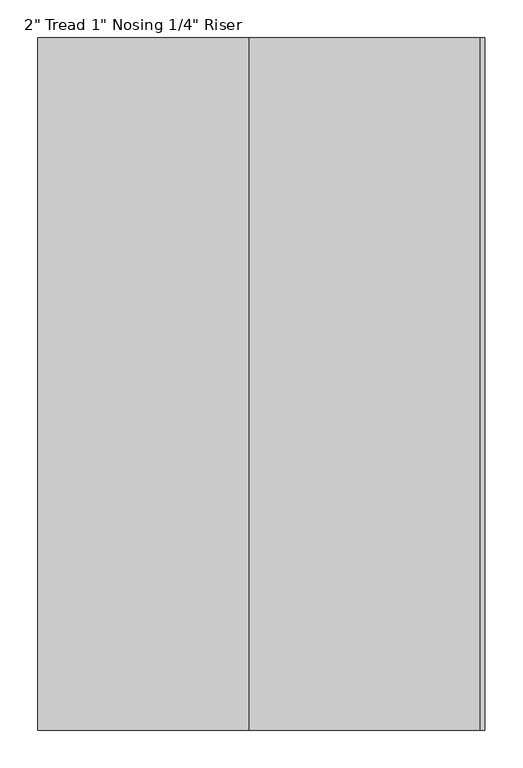
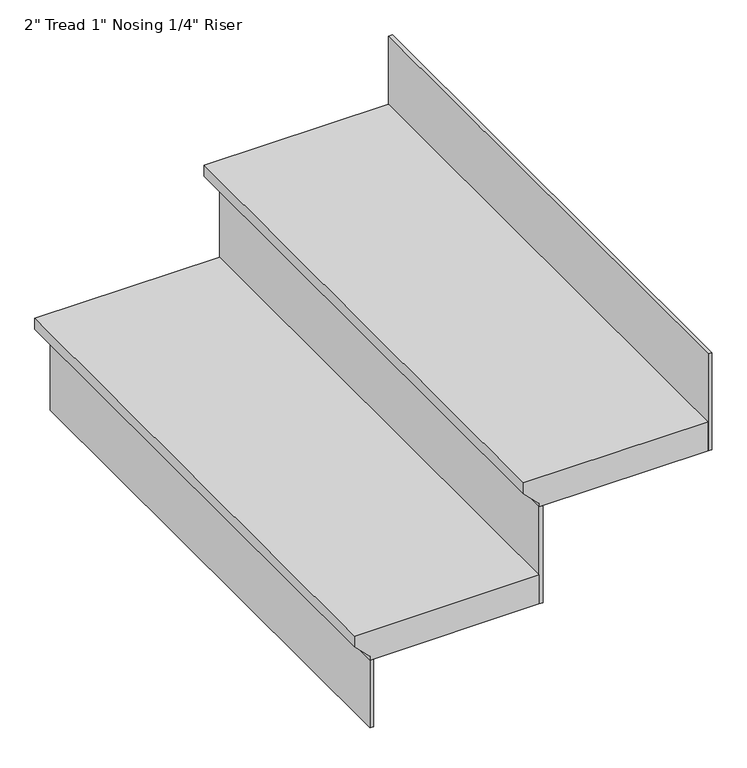
"""IFC4 building model written with IfcOpenShell, lengths in millimetres: stair flight geometry."""

from ifc_helpers import new_model, si_unit, frame, origin, place, context, project, spatial, polyline, outline, extrude, source, transform, mapped, element, save


def stair_flight_c315cc2a(model_context):
    return source(origin(), model_context, "Body", "SweptSolid", [
        extrude(outline(polyline([(2201.3333333, -9510.0836698), (2201.3333333, -9814.8836698), (2182.2833333, -9814.8836698), (2156.8833333, -9789.4836698), (2150.5333333, -9789.4836698), (2150.5333333, -9510.0836698), (2201.3333333, -9510.0836698)])), frame((0.0, -1606.7093225, 0.0), z_axis=(0.0, 1.0, 0.0), x_axis=(0.0, 0.0, 1.0)), (0.0, 0.0, 1.0), 914.4),
        extrude(outline(polyline([(-9783.1336698, -1606.7093225), (-9789.4836698, -1606.7093225), (-9789.4836698, -692.3093225), (-9783.1336698, -692.3093225), (-9783.1336698, -1606.7093225)])), frame((0.0, 0.0, 2032.0), z_axis=(0.0, 0.0, 1.0), x_axis=(1.0, 0.0, 0.0)), (0.0, 0.0, 1.0), 118.5333333),
        extrude(outline(polyline([(-9503.7336698, -1606.7093225), (-9510.0836698, -1606.7093225), (-9510.0836698, -692.3093225), (-9503.7336698, -692.3093225), (-9503.7336698, -1606.7093225)])), frame((0.0, 0.0, 2150.5333333), z_axis=(0.0, 0.0, 1.0), x_axis=(1.0, 0.0, 0.0)), (0.0, 0.0, 1.0), 169.3333333),
        extrude(outline(polyline([(-9224.3336698, -1606.7093225), (-9230.6836698, -1606.7093225), (-9230.6836698, -692.3093225), (-9224.3336698, -692.3093225), (-9224.3336698, -1606.7093225)])), frame((0.0, 0.0, 2319.8666667), z_axis=(0.0, 0.0, 1.0), x_axis=(1.0, 0.0, 0.0)), (0.0, 0.0, 1.0), 169.3333333),
        extrude(outline(polyline([(2370.6666667, -9230.6836698), (2370.6666667, -9535.4836698), (2351.6166667, -9535.4836698), (2326.2166667, -9510.0836698), (2319.8666667, -9510.0836698), (2319.8666667, -9230.6836698), (2370.6666667, -9230.6836698)])), frame((0.0, -1606.7093225, 0.0), z_axis=(0.0, 1.0, 0.0), x_axis=(0.0, 0.0, 1.0)), (0.0, 0.0, 1.0), 914.4),
    ])


if __name__ == "__main__":
    model = new_model("IFC4")
    model_context = context("Model", 3, world=origin())
    ifc_project = project(units=[si_unit("LENGTHUNIT", "METRE", prefix="MILLI")], contexts=[model_context])
    site = spatial("IfcSite", under=ifc_project)
    building = spatial("IfcBuilding", under=site)
    placement = place(None, origin())
    stair_flight_shape = stair_flight_c315cc2a(model_context)
    element("IfcStairFlight", 1, ObjectType="2\" Tread 1\" Nosing 1/4\" Riser", at=placement, inside=building, context=model_context, shape_type="MappedRepresentation", body=[
        mapped(stair_flight_shape, transform((0.0, 0.0, 0.0), x_axis=(1.0, 0.0, 0.0), y_axis=(0.0, 1.0, 0.0), z_axis=(0.0, 0.0, 1.0))),
    ])
    save(model, "model.ifc")
